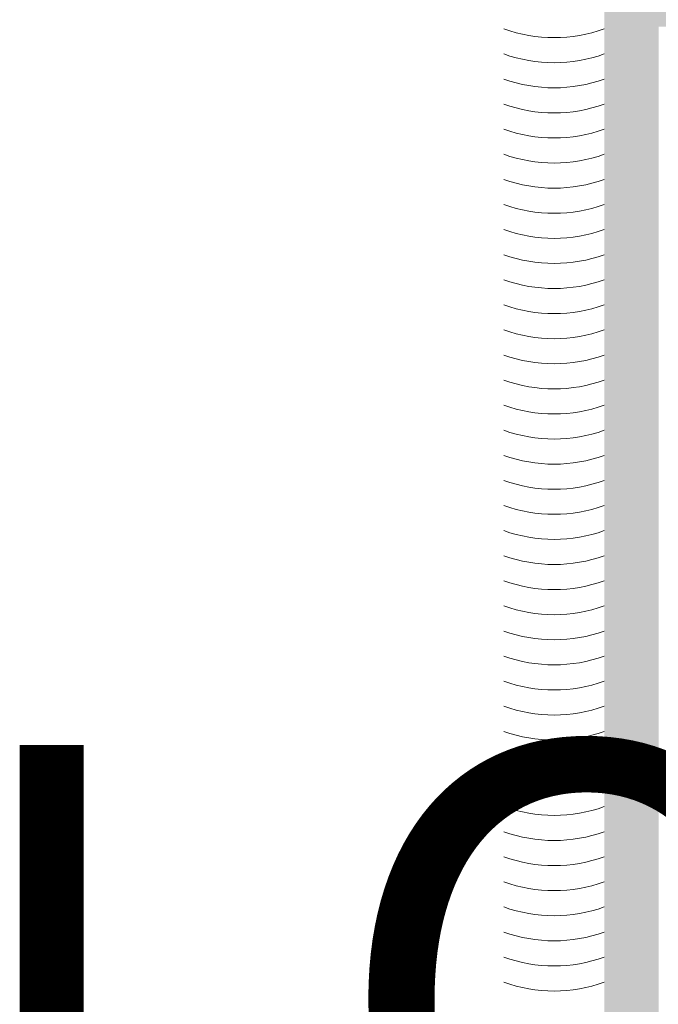
# Model space of a CAD drawing. Units: inches. Extents: x 844 to 2234, y 346 to 1084.
# Tile 74 of 93: x 1989.98 to 1997.48, y 701.36 to 712.93. Entities that reach past the tile are written whole.
import ezdxf

# ---------------------------------------------------------------- set-up
doc = ezdxf.new("R2010")
doc.units = ezdxf.units.IN
doc.header["$MEASUREMENT"] = 0
for name, color, linetype, lineweight in [('A-ANNO-DIMS', 2, 'Continuous', 18), ('furniture', 8, 'Continuous', 18), ('RA-AP-01$0$INT', 35, 'Continuous', 5)]:
    doc.layers.add(name, color=color, linetype=linetype, lineweight=lineweight)
doc.layers.add('RA-AP-01$0$FURN', color=3, linetype='Continuous')
doc.styles.get("Standard").update_dxf_attribs({"font": 'arial.ttf'})
doc.dimstyles.get("Standard").update_dxf_attribs({"dimtxt": 6, "dimasz": 3, "dimexe": 0.18, "dimexo": 0.0625, "dimgap": 0.09, "dimtad": 0, "dimtih": 1, "dimtoh": 1, "dimdec": 1, "dimzin": 0, "dimdsep": 46, "dimlunit": 3, "dimtxsty": 'Standard', "dimblk": 'ARCHTICK', "dimcen": 0.09, "dimadec": 0, "dimazin": 0, "dimtfac": 1, "dimtdec": 1, "dimtofl": 0, "dimtmove": 0, "dimatfit": 3, "dimfxl": 1, "dimtolj": 1, "dimtzin": 0, "dimarcsym": 0})

# ---------------------------------------------------------------- blocks, each defined once
blk = doc.blocks.new('A$C18D01794')
at = {"layer": 'RA-AP-01$0$INT'}
h = blk.add_hatch(color=256, dxfattribs=at)
h.paths.add_polyline_path([(4.35521, -6.15671), (4.35521, -8.05671), (5.45521, -8.05671), (5.45521, -6.15671)])
h.paths.add_polyline_path([(4.40521, -8.00671), (4.40521, -6.20671), (5.40521, -6.20671), (5.40521, -8.00671)], flags=16)
for centre in [(5.50141, -7.25536), (5.50141, -7.27846), (5.50141, -7.30156), (5.50141, -7.32466), (5.50141, -7.34776), (5.50141, -7.37086), (5.50141, -7.39396), (5.50141, -7.41706), (5.50141, -7.44016), (5.50141, -7.46326), (5.50141, -7.48636), (5.50141, -7.50946), (5.50141, -7.53256), (5.50141, -7.55566), (5.50141, -7.57876), (5.50141, -7.60186), (5.50141, -7.62496), (5.50141, -7.64806), (5.50141, -7.67116), (5.50141, -7.67116), (5.50141, -7.69426), (5.50141, -7.71736), (5.50141, -7.74046), (5.50141, -7.76356), (5.50141, -7.78666), (5.50141, -7.80976), (5.50141, -7.83286), (5.50141, -7.85596), (5.50141, -7.87906), (5.50141, -7.90216), (5.50141, -7.92526), (5.50141, -7.94836), (5.50141, -7.97146), (5.50141, -7.99456), (5.50141, -8.01766), (5.50141, -8.04076), (5.50141, -8.06386), (5.50141, -8.08696), (5.50141, -8.11006), (5.50141, -8.13316)]:
    blk.add_arc(centre, 0.13641, 70.20384, 109.79616, dxfattribs=at)
blk = doc.blocks.new('A$C5D2F253E')
at = {"layer": 'RA-AP-01$0$FURN', "xscale": -0.7999999999883585, "yscale": 0.7999999999883585, "zscale": 0.8, "rotation": 90}
blk.add_blockref('A$C18D01794', (-5.68776, 4.75792), dxfattribs=at)
blk = doc.blocks.new('_ArchTick')
at = {"color": 0, "linetype": 'ByBlock', "const_width": 0.15}
blk.add_lwpolyline([(-0.5, -0.5), (0.5, 0.5)], dxfattribs=at)
blk = doc.blocks.new('*D121')
at = {"layer": 'A-ANNO-DIMS', "color": 0, "lineweight": -2, "transparency": 16777216}
for p, q in [((2030.272, 734.263), (2040.245, 734.263)), ((2040.065, 734.263), (2040.065, 704.604)), ((2040.065, 668.557), (2040.065, 698.216)), ((2030.272, 668.557), (2040.245, 668.557))]:
    blk.add_line(p, q, dxfattribs=at)
at = {"layer": 'Defpoints', "color": 0, "transparency": 16777216}
for p in [(2030.209, 734.263), (2040.065, 734.263), (2030.209, 668.557)]:
    blk.add_point(p, dxfattribs=at)
at = {"layer": 'A-ANNO-DIMS', "color": 0, "lineweight": -2, "transparency": 16777216, "xscale": 3, "yscale": 3, "zscale": 3}
for p, rotation in [((2040.065, 734.263), 90), ((2040.065, 668.557), 270)]:
    blk.add_blockref('_ArchTick', p, dxfattribs=dict(at, rotation=rotation))
at = {"layer": 'A-ANNO-DIMS', "color": 0, "transparency": 16777216, "insert": (2040.065, 701.41), "char_height": 6, "attachment_point": 5}
blk.add_mtext('\\A1;LOUNGE SET 5\'-5 1/2" TYP.', dxfattribs=at)

msp = doc.modelspace()

# ---------------------------------------------------------------- block references
at = {"layer": 'furniture', "xscale": -15.94108302203742, "yscale": 15.94108302203742, "zscale": 15.94108302203742, "rotation": 270}
msp.add_blockref('A$C5D2F253E', (1990.567, 701.403), dxfattribs=at)

# ---------------------------------------------------------------- dimensions: what is measured, and where the dimension line sits
at = {"layer": 'A-ANNO-DIMS'}
dim = msp.add_linear_dim(base=(2040.065, 734.263), p1=(2030.209, 668.557), p2=(2030.209, 734.263), angle=90, text='LOUNGE SET <> TYP.', dimstyle='Standard', override={"dimdec": 1, "dimlfac": 1, "dimrnd": 0, "dimzin": 1, "dimdsep": 46, "dimlunit": 4, "dimfrac": 2}, dxfattribs=at)
dim.commit()
dim.dimension.update_dxf_attribs({"geometry": '*D121', "text_midpoint": (2040.065, 701.41)})

doc.saveas('drawing.dxf')
